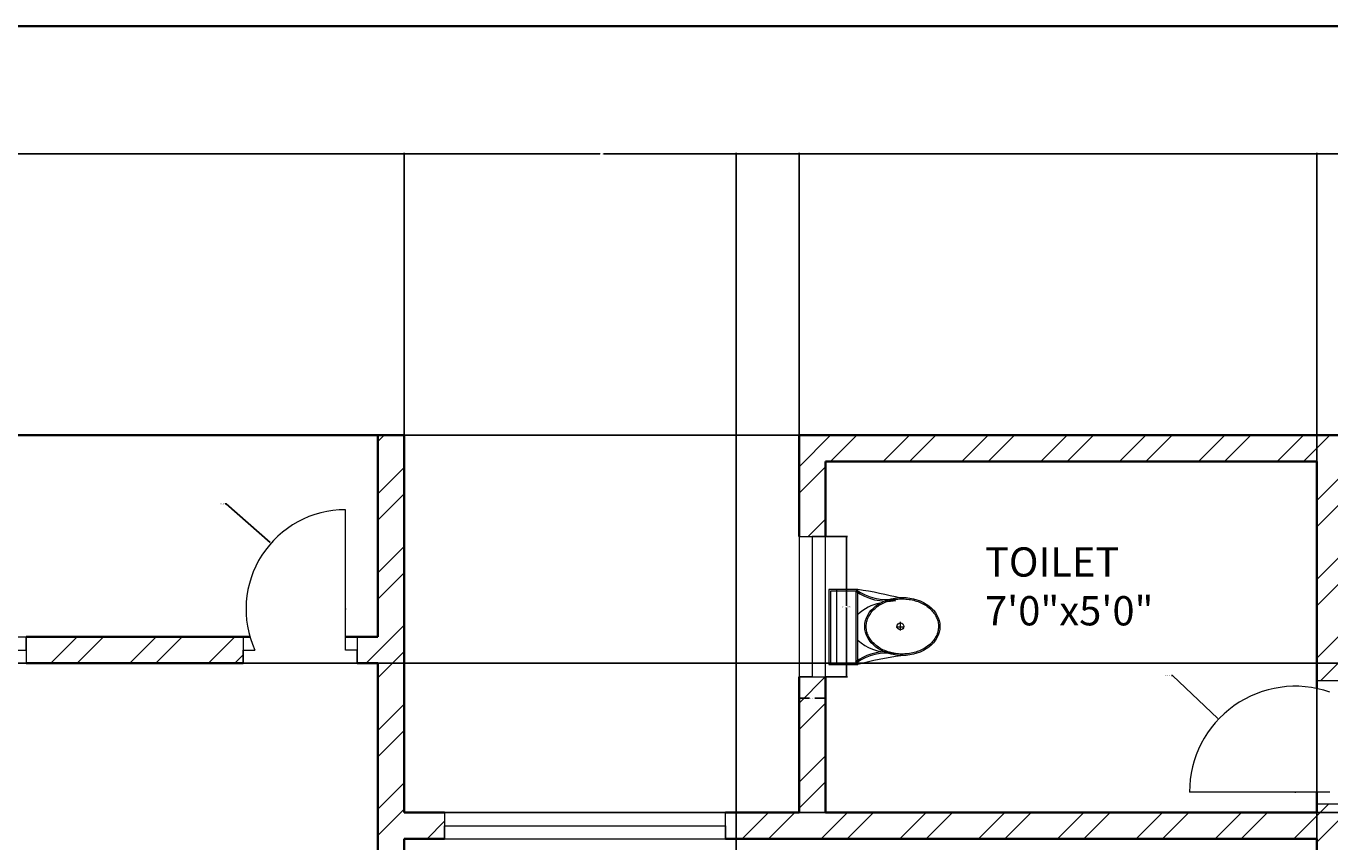
# Model space of a CAD drawing. Units: inches. Extents: x 2008 to 2657, y 1077 to 2165.
# Tile 13 of 16: x 2186 to 2409, y 2025 to 2165. Entities that reach past the tile are written whole.
import ezdxf

# ---------------------------------------------------------------- set-up
doc = ezdxf.new("R2010")
doc.units = ezdxf.units.IN
for name, color, linetype, lineweight in [('A-ANNO-DIMS', 2, 'Continuous', 18), ('A-ANNO-TTLB', 7, 'Continuous', 35), ('A-AREA-IDEN', 4, 'Continuous', 18), ('A-DOOR', 11, 'Continuous', 18), ('A-FLOR-FIXT', 8, 'Continuous', 18), ('A-GLAZ', 191, 'Continuous', 18), ('A-WALL', 7, 'Continuous', 35)]:
    doc.layers.add(name, color=color, linetype=linetype, lineweight=lineweight)
doc.layers.add('A-WALL-PATT', color=30, linetype='Continuous', lineweight=13, true_color=0xf8991e)
doc.styles.get("Standard").update_dxf_attribs({"font": 'arial.ttf'})
doc.dimstyles.get("Standard").update_dxf_attribs({"dimtxt": 0.18, "dimasz": 0.18, "dimexe": 0.18, "dimexo": 0.0625, "dimgap": 0.09, "dimtad": 0, "dimtih": 1, "dimtoh": 1, "dimdec": 4, "dimzin": 0, "dimdsep": 46, "dimtxsty": 'Standard', "dimcen": 0.09, "dimadec": 0, "dimazin": 0, "dimtfac": 1, "dimtdec": 4, "dimtofl": 0, "dimtmove": 0, "dimatfit": 3, "dimfxl": 1, "dimtolj": 1, "dimtzin": 0, "dimarcsym": 0})

# ---------------------------------------------------------------- blocks, each defined once
blk = doc.blocks.new('A$C31115884')
for p, q in [((283.1, 497.7), (223.4, 497.7)), ((257.5, 466.4), (257.5, 523.2)), ((0, 200), (0, 0)), ((520, 200), (0, 200)), ((10, 190), (10, 10)), ((510, 190), (10, 190)), ((510, 10), (510, 190)), ((520, 0), (520, 200)), ((510, 54.5), (0, 54.5)), ((10, 10), (510, 10)), ((0, 0), (520, 0))]:
    blk.add_line(p, q)
blk.add_circle((255.6, 496.4), 23.6)
for centre, radius, start, end in [((2777.7, -204.6), 2807, 165.4549, 171.71327), ((-294.5, 403.3), 364.7, 324.20913, 9.34987), ((-294.5, 403.3), 374.7, 324.20913, 9.34987), ((805.8, 403.3), 364.7, 170.65013, 215.79087), ((3237, 905), 2807, 188.28673, 194.5451), ((139.5, 406.2), 293.5, 315.84364, 2.65635), ((805.8, 403.3), 374.7, 179.20365, 215.79087), ((383.6, 406.2), 293.5, 190.27735, 224.15636)]:
    blk.add_arc(centre, radius, start, end)
blk.add_ellipse((256.2, 509.9), major_axis=(0, -260.7), ratio=0.772727)
blk.add_open_spline([(256.2, 259.2), (263.1, 259.2), (270, 259.7), (287.8, 262.3), (298.7, 265.1), (319.9, 273.1), (330.2, 278.4), (350.1, 291.1), (359.7, 298.7), (377.7, 315.9), (386.2, 325.5), (401.7, 346.6), (408.8, 358.1), (421.3, 382.5), (426.8, 395.5), (435.9, 422.4), (439.5, 436.4), (444.8, 465.1), (446.5, 479.7), (447.9, 509.2), (447.6, 524), (445, 553.3), (442.7, 567.8), (436.3, 596), (432.1, 609.7), (421.9, 636), (416, 648.6), (402.5, 672.1), (395, 683), (378.6, 703), (369.8, 712.1), (351.1, 728), (341.3, 734.8), (320.9, 746.2), (310.4, 750.7), (288.9, 757.3), (278, 759.4), (256, 761), (245, 760.6), (223.1, 757.2), (212.3, 754.3), (191.1, 746.1), (180.8, 740.7), (160.9, 727.8), (151.4, 720.1), (133.5, 702.7), (125.1, 693), (109.6, 671.7), (102.6, 660.2), (90.2, 635.7), (84.9, 622.7), (76, 595.6), (72.4, 581.6), (67.2, 552.9), (65.6, 538.2), (64.4, 508.8), (64.8, 494), (67.5, 464.7), (69.9, 450.2), (76.6, 422), (80.8, 408.3), (91.1, 382.2), (97.2, 369.7), (110.8, 346.3), (118.4, 335.4), (134.8, 315.6), (143.7, 306.7), (162.4, 290.9), (172.3, 284.2), (192.8, 273), (203.3, 268.6), (224.8, 262.2), (235.8, 260.2), (249.9, 259.3), (253, 259.2), (256.2, 259.2)], degree=3, knots=[0, 0, 0, 0, 0.110105, 0.110105, 0.285049, 0.285049, 0.459994, 0.459994, 0.634938, 0.634938, 0.809882, 0.809882, 0.984827, 0.984827, 1.159771, 1.159771, 1.334715, 1.334715, 1.50966, 1.50966, 1.684604, 1.684604, 1.859549, 1.859549, 2.034493, 2.034493, 2.209437, 2.209437, 2.384382, 2.384382, 2.559326, 2.559326, 2.73427, 2.73427, 2.909215, 2.909215, 3.084159, 3.084159, 3.259103, 3.259103, 3.434048, 3.434048, 3.608992, 3.608992, 3.783936, 3.783936, 3.958881, 3.958881, 4.133825, 4.133825, 4.30877, 4.30877, 4.483714, 4.483714, 4.658658, 4.658658, 4.833603, 4.833603, 5.008547, 5.008547, 5.183491, 5.183491, 5.358436, 5.358436, 5.53338, 5.53338, 5.708324, 5.708324, 5.883269, 5.883269, 6.058213, 6.058213, 6.233158, 6.233158, 6.283185, 6.283185, 6.283185, 6.283185])
blk = doc.blocks.new('WIN-60IN-B')
for p, q in [((0, 4.5), (0, 0)), ((0, 4.5), (60, 4.5)), ((60, 2.25), (60, 4.5)), ((60, 4.5), (60, 0)), ((0, 0), (0, 2.25)), ((0, 2.25), (60, 2.25)), ((60, 0), (0, 0))]:
    blk.add_line(p, q)
blk = doc.blocks.new('WIN-24IN-B')
for p, q in [((0, 24), (4.5, 24)), ((0, 24), (0, 0)), ((4.5, 24), (2.25, 24)), ((2.25, 24), (2.25, 0)), ((4.5, 0), (4.5, 24)), ((2.25, 0), (0, 0)), ((0, 0), (4.5, 0))]:
    blk.add_line(p, q)
blk = doc.blocks.new('*D23')
at = {"layer": 'A-ANNO-DIMS', "color": 0, "lineweight": -2, "transparency": 16777216}
for p, q in [((2322.82, 2077.34), (2326.54, 2077.34)), ((2326.36, 2077.16), (2326.36, 2065.52)), ((2326.36, 2053.52), (2326.36, 2065.16)), ((2322.82, 2053.34), (2326.54, 2053.34))]:
    blk.add_line(p, q, dxfattribs=at)
at = {"layer": 'A-ANNO-DIMS', "color": 0, "transparency": 16777216}
for points in [[(2326.33, 2077.16), (2326.39, 2077.16), (2326.36, 2077.34)], [(2326.33, 2053.52), (2326.39, 2053.52), (2326.36, 2053.34)]]:
    blk.add_solid(points, dxfattribs=at)
at = {"layer": 'Defpoints', "color": 0, "transparency": 16777216}
for p in [(2322.76, 2077.34), (2326.36, 2077.34), (2322.76, 2053.34)]:
    blk.add_point(p, dxfattribs=at)
at = {"layer": 'A-ANNO-DIMS', "color": 0, "transparency": 16777216, "insert": (2326.36, 2065.34), "char_height": 0.18, "attachment_point": 5}
blk.add_mtext('\\A1;WIN B 24 TYP.', dxfattribs=at)
blk = doc.blocks.new('*D24')
at = {"layer": 'A-ANNO-DIMS', "color": 0, "lineweight": -2, "transparency": 16777216}
for p, q in [((2318.26, 2053.28), (2318.26, 2049.56)), ((2322.76, 2053.28), (2322.76, 2049.56)), ((2318.44, 2049.74), (2320.05, 2049.74)), ((2322.58, 2049.74), (2320.97, 2049.74))]:
    blk.add_line(p, q, dxfattribs=at)
at = {"layer": 'A-ANNO-DIMS', "color": 0, "transparency": 16777216}
for points in [[(2318.44, 2049.77), (2318.44, 2049.71), (2318.26, 2049.74)], [(2322.58, 2049.77), (2322.58, 2049.71), (2322.76, 2049.74)]]:
    blk.add_solid(points, dxfattribs=at)
at = {"layer": 'Defpoints', "color": 0, "transparency": 16777216}
for p in [(2318.26, 2053.34), (2322.76, 2053.34), (2322.76, 2049.74)]:
    blk.add_point(p, dxfattribs=at)
at = {"layer": 'A-ANNO-DIMS', "color": 0, "transparency": 16777216, "insert": (2320.51, 2049.74), "char_height": 0.18, "attachment_point": 5}
blk.add_mtext('\\A1;5 TYP.', dxfattribs=at)
blk = doc.blocks.new('*D34')
at = {"layer": 'A-ANNO-DIMS', "color": 0, "lineweight": -2, "transparency": 16777216}
for p, q in [((2104.76, 2094.74), (2104.76, 2142.9)), ((2104.94, 2142.72), (2177.48, 2142.72)), ((2250.58, 2142.72), (2178.04, 2142.72)), ((2250.76, 2094.74), (2250.76, 2142.9))]:
    blk.add_line(p, q, dxfattribs=at)
at = {"layer": 'A-ANNO-DIMS', "color": 0, "transparency": 16777216}
for points in [[(2104.94, 2142.75), (2104.94, 2142.69), (2104.76, 2142.72)], [(2250.58, 2142.75), (2250.58, 2142.69), (2250.76, 2142.72)]]:
    blk.add_solid(points, dxfattribs=at)
at = {"layer": 'Defpoints', "color": 0, "transparency": 16777216}
for p in [(2250.76, 2142.72), (2104.76, 2094.67), (2250.76, 2094.67)]:
    blk.add_point(p, dxfattribs=at)
at = {"layer": 'A-ANNO-DIMS', "color": 0, "transparency": 16777216, "insert": (2177.76, 2142.72), "char_height": 0.18, "attachment_point": 5}
blk.add_mtext('\\A1;146', dxfattribs=at)
blk = doc.blocks.new('*D35')
at = {"layer": 'A-ANNO-DIMS', "color": 0, "lineweight": -2, "transparency": 16777216}
for p, q in [((2250.76, 2094.74), (2250.76, 2142.9)), ((2250.94, 2142.72), (2284.19, 2142.72)), ((2318.08, 2142.72), (2284.84, 2142.72)), ((2318.26, 2094.74), (2318.26, 2142.9))]:
    blk.add_line(p, q, dxfattribs=at)
at = {"layer": 'A-ANNO-DIMS', "color": 0, "transparency": 16777216}
for points in [[(2250.94, 2142.75), (2250.94, 2142.69), (2250.76, 2142.72)], [(2318.08, 2142.75), (2318.08, 2142.69), (2318.26, 2142.72)]]:
    blk.add_solid(points, dxfattribs=at)
at = {"layer": 'Defpoints', "color": 0, "transparency": 16777216}
for p in [(2318.26, 2142.72), (2250.76, 2094.67), (2318.26, 2094.67)]:
    blk.add_point(p, dxfattribs=at)
at = {"layer": 'A-ANNO-DIMS', "color": 0, "transparency": 16777216, "insert": (2284.51, 2142.72), "char_height": 0.18, "attachment_point": 5}
blk.add_mtext('\\A1;67.5', dxfattribs=at)
blk = doc.blocks.new('*D36')
at = {"layer": 'A-ANNO-DIMS', "color": 0, "lineweight": -2, "transparency": 16777216}
for p, q in [((2318.26, 2094.74), (2318.26, 2142.9)), ((2318.44, 2142.72), (2364.54, 2142.72)), ((2411.08, 2142.72), (2364.98, 2142.72)), ((2411.26, 2094.74), (2411.26, 2142.9))]:
    blk.add_line(p, q, dxfattribs=at)
at = {"layer": 'A-ANNO-DIMS', "color": 0, "transparency": 16777216}
for points in [[(2318.44, 2142.75), (2318.44, 2142.69), (2318.26, 2142.72)], [(2411.08, 2142.75), (2411.08, 2142.69), (2411.26, 2142.72)]]:
    blk.add_solid(points, dxfattribs=at)
at = {"layer": 'Defpoints', "color": 0, "transparency": 16777216}
for p in [(2411.26, 2142.72), (2318.26, 2094.67), (2411.26, 2094.67)]:
    blk.add_point(p, dxfattribs=at)
at = {"layer": 'A-ANNO-DIMS', "color": 0, "transparency": 16777216, "insert": (2364.76, 2142.72), "char_height": 0.18, "attachment_point": 5}
blk.add_mtext('\\A1;93', dxfattribs=at)
blk = doc.blocks.new('*D49')
at = {"layer": 'A-ANNO-DIMS', "color": 0, "lineweight": -2, "transparency": 16777216}
for p, q in [((2250.82, 2094.67), (2624.99, 2094.67)), ((2624.81, 2094.49), (2624.81, 2062.61)), ((2624.81, 2030.35), (2624.81, 2062.24)), ((2250.82, 2030.17), (2624.99, 2030.17))]:
    blk.add_line(p, q, dxfattribs=at)
at = {"layer": 'A-ANNO-DIMS', "color": 0, "transparency": 16777216}
for points in [[(2624.78, 2094.49), (2624.84, 2094.49), (2624.81, 2094.67)], [(2624.78, 2030.35), (2624.84, 2030.35), (2624.81, 2030.17)]]:
    blk.add_solid(points, dxfattribs=at)
at = {"layer": 'Defpoints', "color": 0, "transparency": 16777216}
for p in [(2250.76, 2094.67), (2624.81, 2094.67), (2250.76, 2030.17)]:
    blk.add_point(p, dxfattribs=at)
at = {"layer": 'A-ANNO-DIMS', "color": 0, "transparency": 16777216, "insert": (2624.81, 2062.42), "char_height": 0.18, "attachment_point": 5}
blk.add_mtext('\\A1;64.5', dxfattribs=at)
blk = doc.blocks.new('*D51')
at = {"layer": 'A-ANNO-DIMS', "color": 0, "lineweight": -2, "transparency": 16777216}
for p, q in [((2307.5, 1617.74), (2307.5, 2142.9)), ((2307.68, 2142.72), (2356.74, 2142.72)), ((2406.58, 2142.72), (2357.53, 2142.72)), ((2406.76, 1617.74), (2406.76, 2142.9))]:
    blk.add_line(p, q, dxfattribs=at)
at = {"layer": 'A-ANNO-DIMS', "color": 0, "transparency": 16777216}
for points in [[(2307.68, 2142.75), (2307.68, 2142.69), (2307.5, 2142.72)], [(2406.58, 2142.75), (2406.58, 2142.69), (2406.76, 2142.72)]]:
    blk.add_solid(points, dxfattribs=at)
at = {"layer": 'Defpoints', "color": 0, "transparency": 16777216}
for p in [(2406.76, 2142.72), (2307.5, 1617.67), (2406.76, 1617.67)]:
    blk.add_point(p, dxfattribs=at)
at = {"layer": 'A-ANNO-DIMS', "color": 0, "transparency": 16777216, "insert": (2357.13, 2142.72), "char_height": 0.18, "attachment_point": 5}
blk.add_mtext('\\A1;99.26', dxfattribs=at)
blk = doc.blocks.new('*D66')
at = {"layer": 'A-ANNO-DIMS', "color": 0, "lineweight": -2, "transparency": 16777216}
for p, q in [((2572.2, 2055.67), (2028.03, 2055.67)), ((2028.21, 2055.49), (2028.21, 2025.16)), ((2028.21, 1994.47), (2028.21, 2024.8)), ((2572.2, 1994.29), (2028.03, 1994.29))]:
    blk.add_line(p, q, dxfattribs=at)
at = {"layer": 'A-ANNO-DIMS', "color": 0, "transparency": 16777216}
for points in [[(2028.18, 2055.49), (2028.24, 2055.49), (2028.21, 2055.67)], [(2028.18, 1994.47), (2028.24, 1994.47), (2028.21, 1994.29)]]:
    blk.add_solid(points, dxfattribs=at)
at = {"layer": 'Defpoints', "color": 0, "transparency": 16777216}
for p in [(2572.26, 2055.67), (2028.21, 1994.29), (2572.26, 1994.29)]:
    blk.add_point(p, dxfattribs=at)
at = {"layer": 'A-ANNO-DIMS', "color": 0, "transparency": 16777216, "insert": (2028.21, 2024.98), "char_height": 0.18, "attachment_point": 5}
blk.add_mtext('\\A1;61.39', dxfattribs=at)
blk = doc.blocks.new('*D85')
at = {"layer": 'A-ANNO-DIMS', "color": 0, "lineweight": -2, "transparency": 16777216}
for p, q in [((2220.17, 2082.93), (2220.35, 2082.93)), ((2220.35, 2082.93), (2227.86, 2076.3)), ((2240.63, 2064.94), (2240.81, 2064.94)), ((2240.72, 2064.85), (2240.72, 2065.03))]:
    blk.add_line(p, q, dxfattribs=at)
at = {"layer": 'A-ANNO-DIMS', "color": 0, "transparency": 16777216}
blk.add_solid([(2227.88, 2076.33), (2227.84, 2076.28), (2227.99, 2076.18)], dxfattribs=at)
at = {"layer": 'Defpoints', "color": 0, "transparency": 16777216}
for p in [(2227.99, 2076.18), (2240.72, 2064.94)]:
    blk.add_point(p, dxfattribs=at)
at = {"layer": 'A-ANNO-DIMS', "color": 0, "transparency": 16777216, "insert": (2219.69, 2082.93), "char_height": 0.18, "attachment_point": 5}
blk.add_mtext('\\A1;R16.99', dxfattribs=at)
blk = doc.blocks.new('*D86')
at = {"layer": 'A-ANNO-DIMS', "color": 0, "lineweight": -2, "transparency": 16777216}
for p, q in [((2381.93, 2053.59), (2382.11, 2053.59)), ((2382.11, 2053.59), (2389.85, 2046.24)), ((2403, 2033.67), (2403.18, 2033.67)), ((2403.09, 2033.58), (2403.09, 2033.76))]:
    blk.add_line(p, q, dxfattribs=at)
at = {"layer": 'A-ANNO-DIMS', "color": 0, "transparency": 16777216}
blk.add_solid([(2389.87, 2046.27), (2389.83, 2046.22), (2389.98, 2046.12)], dxfattribs=at)
at = {"layer": 'Defpoints', "color": 0, "transparency": 16777216}
for p in [(2389.98, 2046.12), (2403.09, 2033.67)]:
    blk.add_point(p, dxfattribs=at)
at = {"layer": 'A-ANNO-DIMS', "color": 0, "transparency": 16777216, "insert": (2381.38, 2053.59), "char_height": 0.18, "attachment_point": 5}
blk.add_mtext('\\A1;R18.076', dxfattribs=at)

msp = doc.modelspace()

# ---------------------------------------------------------------- hatches: boundary and pattern name
at = {"layer": 'A-WALL-PATT'}
h = msp.add_hatch(dxfattribs=at)
h.set_pattern_fill('ANSI32', color=256)
h.paths.add_polyline_path([(2109.2619, 2094.6743), (2104.7619, 2094.6743), (2104.7619, 2072.1743), (2104.7619, 2021.6151), (2109.2619, 2021.6151), (2109.2619, 2055.6743), (2126.1387, 2055.6743), (2126.1387, 2057.9243), (2126.1387, 2060.1743), (2109.2619, 2060.1743)])
h.paths.add_polyline_path([(2223.2494, 2057.9243), (2223.2494, 2060.1743), (2186.1387, 2060.1743), (2186.1387, 2055.6743), (2223.2494, 2055.6743)])
h.paths.add_polyline_path([(2250.7619, 2072.1743), (2250.7619, 2090.1743), (2250.7619, 2094.6743), (2246.2619, 2094.6743), (2246.2619, 2060.1743), (2242.7242, 2060.1743), (2242.7242, 2055.6743), (2246.2619, 2055.6743), (2246.2619, 1899.6743), (2242.7458, 1899.6743), (2242.7458, 1897.4243), (2242.7458, 1895.1743), (2246.2619, 1895.1743), (2246.2619, 1878.8745), (2248.5119, 1878.8745), (2250.7619, 1878.8745), (2250.7619, 1991.1743), (2250.7619, 2025.6743), (2257.6798, 2025.6743), (2257.6798, 2027.9243), (2257.6798, 2030.1743), (2250.7619, 2030.1743)])
h.paths.add_polyline_path([(2411.2619, 2031.6743), (2409.0119, 2031.6743), (2406.7619, 2031.6743), (2406.7619, 2030.1743), (2322.7619, 2030.1743), (2322.7619, 2053.3443), (2318.2619, 2053.3443), (2318.2619, 2030.1743), (2305.6798, 2030.1743), (2305.6798, 2025.6743), (2318.2619, 2025.6743), (2322.7619, 2025.6743), (2406.7619, 2025.6743), (2406.7619, 1995.6743), (2406.7619, 1847.2677), (2250.7619, 1847.2677), (2250.7619, 1850.9902), (2248.5119, 1850.9902), (2246.2619, 1850.9902), (2246.2619, 1847.1743), (2246.2619, 1842.7677), (2303.0015, 1842.7677), (2303.0015, 1667.2413), (2298.4208, 1667.2413), (2298.4208, 1662.7413), (2303.0015, 1662.7413), (2303.0015, 1649.8758), (2307.5015, 1649.8758), (2307.5015, 1842.7677), (2406.7619, 1842.7677), (2411.2619, 1842.7677), (2411.2619, 1878.6743), (2415.8196, 1878.6743), (2415.8196, 1880.9243), (2415.8196, 1883.1743), (2411.2619, 1883.1743)])
h.paths.add_polyline_path([(2411.2619, 2094.6743), (2406.7619, 2094.6743), (2318.2619, 2094.6743), (2318.2619, 2077.3443), (2322.7619, 2077.3443), (2322.7619, 2090.1743), (2406.7619, 2090.1743), (2406.7619, 2072.1743), (2406.7619, 2067.6743), (2406.7619, 2052.7524), (2411.2619, 2052.7524), (2411.2619, 2055.6743), (2414.9888, 2055.6743), (2414.9888, 2057.9243), (2414.9888, 2060.1743), (2411.2619, 2060.1743), (2411.2619, 2072.1743)])
h.paths.add_polyline_path([(2576.7619, 2072.1743), (2576.7619, 2094.6743), (2572.2619, 2094.6743), (2572.2619, 2060.1743), (2525.8113, 2060.1743), (2525.8113, 2055.6743), (2572.2619, 2055.6743), (2572.2619, 1994.289), (2576.7619, 1994.289)])
h.paths.add_polyline_path([(2465.8113, 2060.1743), (2436.2802, 2060.1743), (2436.2802, 2055.6743), (2465.8113, 2055.6743), (2465.8113, 2057.9243)])
h.paths.add_polyline_path([(2576.7619, 1934.289), (2574.5119, 1934.289), (2572.2619, 1934.289), (2572.2619, 1883.1743), (2447.7027, 1883.1743), (2447.7027, 1878.6743), (2459.7619, 1878.6743), (2459.7619, 1830.4982), (2464.2619, 1830.4982), (2464.2619, 1878.6743), (2572.2619, 1878.6743), (2572.2619, 1868.4883), (2576.7619, 1868.4883)])
h.paths.add_polyline_path([(2576.7619, 1832.4883), (2572.2619, 1832.4883), (2572.2619, 1806.6743), (2464.2619, 1806.6743), (2464.2619, 1809.6629), (2459.7619, 1809.6629), (2459.7619, 1802.1743), (2483.7619, 1802.1743), (2483.7619, 1778.1743), (2488.2619, 1778.1743), (2488.2619, 1802.1743), (2572.2619, 1802.1743), (2572.2619, 1793.6101), (2576.7619, 1793.6101)])
h.paths.add_polyline_path([(2576.7619, 1769.6101), (2572.2619, 1769.6101), (2572.2619, 1754.1743), (2488.2619, 1754.1743), (2488.2619, 1757.2675), (2486.0119, 1757.2675), (2483.7619, 1757.2675), (2483.7619, 1754.1743), (2447.4528, 1754.1743), (2447.4528, 1749.6743), (2483.7619, 1749.6743), (2572.2619, 1749.6743), (2572.2619, 1715.1837), (2576.7619, 1715.1837)])
h.paths.add_polyline_path([(2576.7619, 1655.1837), (2572.2619, 1655.1837), (2572.2619, 1617.6743), (2411.2619, 1617.6743), (2411.2619, 1749.6743), (2414.2827, 1749.6743), (2414.2827, 1754.1743), (2406.7619, 1754.1743), (2406.7619, 1749.6743), (2406.7619, 1617.6743), (2307.5015, 1617.6743), (2307.5015, 1621.0007), (2305.2515, 1621.0007), (2303.0015, 1621.0007), (2303.0015, 1609.6944), (2307.5015, 1609.6944), (2307.5015, 1613.1743), (2406.7619, 1613.1743), (2406.7619, 1476.6743), (2415.532, 1476.6743), (2415.532, 1478.9243), (2415.532, 1481.1743), (2411.2619, 1481.1743), (2411.2619, 1613.1743), (2572.2619, 1613.1743), (2572.2619, 1584.6086), (2576.7619, 1584.6086)])
h.paths.add_polyline_path([(2576.7619, 1524.6086), (2572.2619, 1524.6086), (2572.2619, 1481.1743), (2483.7619, 1481.1743), (2447.5119, 1481.1743), (2447.5119, 1476.6743), (2483.7619, 1476.6743), (2483.7619, 1473.5051), (2488.2619, 1473.5051), (2488.2619, 1476.6743), (2572.2619, 1476.6743), (2572.2619, 1469.5488), (2576.7619, 1469.5488)])
h.paths.add_polyline_path([(2576.7619, 1445.5488), (2572.2619, 1445.5488), (2572.2619, 1428.6743), (2488.2619, 1428.6743), (2488.2619, 1455.6743), (2486.0119, 1455.6743), (2483.7619, 1455.6743), (2483.7619, 1428.6743), (2459.7619, 1428.6743), (2459.7619, 1422.1519), (2464.2619, 1422.1519), (2464.2619, 1424.1743), (2572.2619, 1424.1743), (2572.2619, 1407.5685), (2576.7619, 1407.5685)])
h.paths.add_polyline_path([(2576.7619, 1371.5685), (2572.2619, 1371.5685), (2572.2619, 1352.1743), (2464.2619, 1352.1743), (2464.2619, 1403.1384), (2462.0119, 1403.1384), (2459.7619, 1403.1384), (2459.7619, 1352.1743), (2446.3194, 1352.1743), (2446.3194, 1347.6743), (2572.2619, 1347.6743), (2572.2619, 1321.0291), (2576.7619, 1321.0291)])
h.paths.add_polyline_path([(2462.703, 1227.6743), (2436.0298, 1227.6743), (2436.0298, 1225.4243), (2436.0298, 1223.1743), (2462.703, 1223.1743), (2462.703, 1225.4243)])
h.paths.add_polyline_path([(2576.7619, 1261.0291), (2574.5119, 1261.0291), (2572.2619, 1261.0291), (2572.2619, 1227.6743), (2522.703, 1227.6743), (2522.703, 1223.1743), (2572.2619, 1223.1743), (2572.2619, 1188.6743), (2576.7619, 1188.6743), (2576.7619, 1193.1743), (2576.7619, 1223.1743)])
h.paths.add_polyline_path([(2414.2823, 1227.6743), (2411.2619, 1227.6743), (2411.2619, 1267.1779), (2409.0119, 1267.1779), (2406.7619, 1267.1779), (2406.7619, 1227.6743), (2322.7619, 1227.6743), (2322.7619, 1244.3623), (2318.2619, 1244.3623), (2318.2619, 1223.1743), (2406.7619, 1223.1743), (2406.7619, 1193.1743), (2406.7619, 1188.6743), (2411.2619, 1188.6743), (2411.2619, 1193.1743), (2411.2619, 1223.1743), (2414.2823, 1223.1743)])
h.paths.add_polyline_path([(2411.2619, 1347.6743), (2414.702, 1347.6743), (2414.702, 1349.9243), (2414.702, 1352.1743), (2411.2619, 1352.1743), (2411.2619, 1416.7413), (2307.5015, 1416.7413), (2307.5015, 1579.8489), (2305.2515, 1579.8489), (2303.0015, 1579.8489), (2303.0015, 1566.7413), (2299.2719, 1566.7413), (2299.2719, 1562.2413), (2303.0015, 1562.2413), (2303.0015, 1416.7413), (2246.2619, 1416.7413), (2246.2619, 1409.8616), (2250.7619, 1409.8616), (2250.7619, 1412.2413), (2406.7619, 1412.2413), (2406.7619, 1292.1743), (2304.9703, 1292.1743), (2304.9703, 1287.6743), (2318.2619, 1287.6743), (2318.2619, 1268.3623), (2322.7619, 1268.3623), (2322.7619, 1287.6743), (2406.7619, 1287.6743), (2406.7619, 1285.4748), (2411.2619, 1285.4748)])
h.paths.add_polyline_path([(2109.2619, 1262.7482), (2104.7619, 1262.7482), (2104.7619, 1223.1743), (2104.7619, 1193.1743), (2104.7619, 1188.6743), (2109.2619, 1188.6743), (2109.2619, 1223.1743), (2126.7928, 1223.1743), (2126.7928, 1225.4243), (2126.7928, 1227.6743), (2109.2619, 1227.6743)])
h.paths.add_polyline_path([(2222.3268, 1227.6743), (2186.7928, 1227.6743), (2186.7928, 1223.1743), (2222.3268, 1223.1743)])
h.paths.add_polyline_path([(2250.7619, 1287.6743), (2256.9703, 1287.6743), (2256.9703, 1289.9243), (2256.9703, 1292.1743), (2250.7619, 1292.1743), (2250.7619, 1382.2078), (2248.5119, 1382.2078), (2246.2619, 1382.2078), (2246.2619, 1347.6743), (2246.2619, 1227.6743), (2242.6068, 1227.6743), (2242.6068, 1223.1743), (2246.2619, 1223.1743), (2246.2619, 1188.6743), (2250.7619, 1188.6743), (2250.7619, 1193.1743), (2250.7619, 1227.6743)])
h.paths.add_polyline_path([(2133.2619, 1349.9243), (2133.2619, 1352.1743), (2109.2619, 1352.1743), (2109.2619, 1375.2826), (2104.7619, 1375.2826), (2104.7619, 1322.7482), (2109.2619, 1322.7482), (2109.2619, 1347.6743), (2133.2619, 1347.6743)])
h.paths.add_polyline_path([(2210.2105, 1352.1743), (2161.7619, 1352.1743), (2161.7619, 1412.2413), (2185.7619, 1412.2413), (2185.7619, 1420.1851), (2183.5119, 1420.1851), (2181.2619, 1420.1851), (2181.2619, 1416.7413), (2109.2619, 1416.7413), (2109.2619, 1452.4006), (2104.7619, 1452.4006), (2104.7619, 1399.2826), (2109.2619, 1399.2826), (2109.2619, 1412.2413), (2157.2619, 1412.2413), (2157.2619, 1352.1743), (2154.3383, 1352.1743), (2154.3383, 1347.6743), (2210.2105, 1347.6743)])
h.paths.add_polyline_path([(2185.7619, 1514.2413), (2161.7619, 1514.2413), (2161.7619, 1518.1307), (2159.5119, 1518.1307), (2157.2619, 1518.1307), (2157.2619, 1514.2413), (2109.2619, 1514.2413), (2109.2619, 1528.997), (2107.0119, 1528.997), (2104.7619, 1528.997), (2104.7619, 1488.4006), (2109.2619, 1488.4006), (2109.2619, 1509.7413), (2181.2619, 1509.7413), (2181.2619, 1441.2042), (2185.7619, 1441.2042)])
h.paths.add_polyline_path([(2270.4025, 1566.7413), (2109.2619, 1566.7413), (2080.7619, 1566.7413), (2080.7619, 1586.5643), (2076.2619, 1586.5643), (2076.2619, 1562.2413), (2080.7619, 1562.2413), (2104.7619, 1562.2413), (2104.7619, 1552.997), (2109.2619, 1552.997), (2109.2619, 1562.2413), (2157.2619, 1562.2413), (2157.2619, 1538.2413), (2161.7619, 1538.2413), (2161.7619, 1562.2413), (2205.2619, 1562.2413), (2270.4025, 1562.2413)])
h.paths.add_polyline_path([(2131.6813, 1897.4243), (2131.6813, 1899.6743), (2109.2619, 1899.6743), (2109.2619, 1961.6151), (2104.7619, 1961.6151), (2104.7619, 1886.8042), (2109.2619, 1886.8042), (2109.2619, 1895.1743), (2131.6813, 1895.1743)])
h.paths.add_polyline_path([(2185.7619, 1847.1743), (2161.7619, 1847.1743), (2161.7619, 1895.1743), (2185.7619, 1895.1743), (2211.543, 1895.1743), (2211.543, 1897.4243), (2211.543, 1899.6743), (2154.0916, 1899.6743), (2154.0916, 1897.4243), (2154.0916, 1895.1743), (2157.2619, 1895.1743), (2157.2619, 1847.1743), (2109.2619, 1847.1743), (2109.2619, 1862.8042), (2104.7619, 1862.8042), (2104.7619, 1821.243), (2109.2619, 1821.243), (2109.2619, 1842.6743), (2181.2619, 1842.6743), (2181.2619, 1840.6763), (2185.7619, 1840.6763)])
h.paths.add_polyline_path([(2109.2619, 1785.243), (2104.7619, 1785.243), (2104.7619, 1715.4691), (2109.2619, 1715.4691), (2109.2619, 1730.8423), (2157.2619, 1730.8423), (2157.2619, 1727.6404), (2161.7619, 1727.6404), (2161.7619, 1730.8423), (2185.7619, 1730.8423), (2185.7619, 1822.1438), (2183.5119, 1822.1438), (2181.2619, 1822.1438), (2181.2619, 1735.3423), (2109.2619, 1735.3423)])
h.paths.add_polyline_path([(2109.2619, 1691.4691), (2104.7619, 1691.4691), (2104.7619, 1667.2413), (2076.2619, 1667.2413), (2076.2619, 1646.5643), (2080.7619, 1646.5643), (2080.7619, 1662.7413), (2109.2619, 1662.7413), (2271.4941, 1662.7413), (2271.4941, 1664.9913), (2271.4941, 1667.2413), (2181.2619, 1667.2413), (2161.7619, 1667.2413), (2161.7619, 1708.3752), (2159.5119, 1708.3752), (2157.2619, 1708.3752), (2157.2619, 1667.2413), (2109.2619, 1667.2413)])
h.paths.add_polyline_path([(2233.1467, 1747.4973), (2270.0737, 1747.4973), (2270.0737, 1766.1547), (2233.1467, 1766.1547)], flags=9)

# ---------------------------------------------------------------- linework, layer by layer
at = {"layer": 'A-ANNO-TTLB'}
msp.add_lwpolyline([(2008.4537, 2164.5615), (2657.4477, 2164.5615), (2657.4477, 1076.8888), (2008.4537, 1076.8888)], close=True, dxfattribs=at)
at = {"layer": 'A-DOOR'}
for p, q in [((2240.7242, 2057.9243), (2240.7242, 2081.9243)), ((2223.2494, 2060.1743), (2223.2494, 2055.6743)), ((2242.7242, 2060.1743), (2242.7242, 2055.6743)), ((2223.2494, 2055.6743), (2223.2494, 2057.9243)), ((2223.2494, 2057.9243), (2225.2494, 2057.9243)), ((2242.7242, 2057.9243), (2240.7242, 2057.9243)), ((2242.7242, 2055.6743), (2242.7242, 2057.9243)), ((2406.7619, 2052.7524), (2411.2619, 2052.7524)), ((2409.0119, 2033.6743), (2385.0119, 2033.6743)), ((2406.7619, 2031.6743), (2411.2619, 2031.6743))]:
    msp.add_line(p, q, dxfattribs=at)
for centre, radius, start, end in [((2240.7242, 2064.9354), 16.989, 90, 204.373471), ((2403.0881, 2033.6743), 18.0762, 70.87007, 180)]:
    msp.add_arc(centre, radius, start, end, dxfattribs=at)
at = {"layer": 'A-GLAZ'}
for p, q in [((2257.6798, 2030.1743), (2257.6798, 2025.6743)), ((2305.6798, 2030.1743), (2257.6798, 2030.1743)), ((2305.6798, 2025.6743), (2305.6798, 2030.1743)), ((2257.6798, 2025.6743), (2257.6798, 2027.9243)), ((2257.6798, 2027.9243), (2305.6798, 2027.9243)), ((2305.6798, 2027.9243), (2305.6798, 2025.6743)), ((2257.6798, 2025.6743), (2305.6798, 2025.6743))]:
    msp.add_line(p, q, dxfattribs=at)
at = {"layer": 'A-WALL'}
for p, q in [((2250.7619, 2094.6743), (2104.7619, 2094.6743)), ((2246.2619, 2094.6743), (2246.2619, 2060.1743)), ((2250.7619, 2094.6743), (2246.2619, 2094.6743)), ((2250.7619, 2090.1743), (2250.7619, 2094.6743)), ((2406.7619, 2094.6743), (2318.2619, 2094.6743)), ((2318.2619, 2077.3443), (2318.2619, 2094.6743)), ((2406.7619, 2094.6743), (2572.2619, 2094.6743)), ((2250.7619, 2072.1743), (2250.7619, 2090.1743)), ((2322.7619, 2090.1743), (2322.7619, 2077.3443)), ((2322.7619, 2090.1743), (2406.7619, 2090.1743)), ((2406.7619, 2072.1743), (2406.7619, 2090.1743)), ((2246.2619, 2072.1743), (2246.2619, 2060.1743)), ((2250.7619, 2072.1743), (2250.7619, 2030.1743)), ((2406.7619, 2067.6743), (2406.7619, 2072.1743)), ((2406.7619, 2067.6743), (2406.7619, 2051.3733)), ((2186.1387, 2060.1743), (2224.416, 2060.1743)), ((2240.7242, 2060.1743), (2246.2619, 2060.1743)), ((2186.1387, 2055.6743), (2223.2494, 2055.6743)), ((2242.7242, 2055.6743), (2246.2619, 2055.6743)), ((2246.2619, 2055.6743), (2246.2619, 1899.6743)), ((2318.2619, 2030.1743), (2318.2619, 2053.3443)), ((2322.7619, 2053.3443), (2322.7619, 2030.1743)), ((2406.7619, 2033.6743), (2406.7619, 2030.1743)), ((2257.6798, 2030.1743), (2250.7619, 2030.1743)), ((2318.2619, 2030.1743), (2305.6798, 2030.1743)), ((2322.7619, 2030.1743), (2406.7619, 2030.1743)), ((2250.7619, 2025.6743), (2250.7619, 1877.7035)), ((2257.6798, 2025.6743), (2250.7619, 2025.6743)), ((2318.2619, 2025.6743), (2305.6798, 2025.6743)), ((2322.7619, 2025.6743), (2318.2619, 2025.6743)), ((2406.7619, 2025.6743), (2322.7619, 2025.6743)), ((2406.7619, 2025.6743), (2406.7619, 1995.6743))]:
    msp.add_line(p, q, dxfattribs=at)

# ---------------------------------------------------------------- block references
at = {"layer": 'A-FLOR-FIXT', "xscale": 0.0246256636748975, "yscale": 0.0246256636748975, "zscale": 0.0246256636748975, "rotation": 270}
msp.add_blockref('A$C31115884', (2323.3687, 2068.2761), dxfattribs=at)
at = {"layer": 'A-GLAZ'}
for name, p in [('WIN-24IN-B', (2318.262, 2053.344)), ('WIN-60IN-B', (2126.139, 2055.674))]:
    msp.add_blockref(name, p, dxfattribs=at)

# ---------------------------------------------------------------- texts
at = {"layer": 'A-AREA-IDEN', "insert": (2350.0509, 2075.4874), "char_height": 5, "attachment_point": 1}
msp.add_mtext_dynamic_manual_height_columns('TOILET\\P7\'0"x5\'0"', width=100.78829, gutter_width=12.5, heights=[0], dxfattribs=at)

# ---------------------------------------------------------------- dimensions: what is measured, and where the dimension line sits
at = {"layer": 'A-ANNO-DIMS'}
for base, p1, p2, override, picture, middle in [((2250.7619, 2142.7243), (2104.7619, 2094.6743), (2250.7619, 2094.6743), {"dimdec": 0, "dimlfac": 1, "dimrnd": 0, "dimzin": 0, "dimdsep": 46, "dimlunit": 2}, '*D34', (2177.7619, 2142.7243)), ((2318.2619, 2142.7243), (2250.7619, 2094.6743), (2318.2619, 2094.6743), {"dimdec": 1, "dimlfac": 1, "dimrnd": 0, "dimzin": 0, "dimdsep": 46, "dimlunit": 2}, '*D35', (2284.5119, 2142.7243)), ((2406.7619, 2142.7243), (2307.5015, 1617.6743), (2406.7619, 1617.6743), {"dimdec": 2, "dimlfac": 1, "dimrnd": 0, "dimzin": 0, "dimdsep": 46, "dimlunit": 2}, '*D51', (2357.1317, 2142.7243)), ((2411.2619, 2142.7243), (2318.2619, 2094.6743), (2411.2619, 2094.6743), {"dimdec": 0, "dimlfac": 1, "dimrnd": 0, "dimzin": 0, "dimdsep": 46, "dimlunit": 2}, '*D36', (2364.7619, 2142.7243))]:
    dim = msp.add_linear_dim(base=base, p1=p1, p2=p2, dimstyle='Standard', override=override, dxfattribs=at)
    dim.commit()
    dim.dimension.update_dxf_attribs({"geometry": picture, "text_midpoint": middle})
for base, p1, p2, override, picture, middle in [((2624.8119, 2094.6743), (2250.7619, 2030.1743), (2250.7619, 2094.6743), {"dimdec": 1, "dimlfac": 1, "dimrnd": 0, "dimzin": 0, "dimdsep": 46, "dimlunit": 2}, '*D49', (2624.8119, 2062.4243)), ((2028.2119, 1994.289), (2572.2619, 2055.6743), (2572.2619, 1994.289), {"dimdec": 2, "dimlfac": 1, "dimrnd": 0, "dimzin": 0, "dimdsep": 46, "dimlunit": 2}, '*D66', (2028.2119, 2024.9817))]:
    dim = msp.add_linear_dim(base=base, p1=p1, p2=p2, angle=90, dimstyle='Standard', override=override, dxfattribs=at)
    dim.commit()
    dim.dimension.update_dxf_attribs({"geometry": picture, "text_midpoint": middle})
for center, mpoint, override, picture, middle in [((2240.7242, 2064.9354), (2227.9922, 2076.1835), {"dimdec": 2, "dimlfac": 1, "dimrnd": 0, "dimzin": 0, "dimdsep": 46, "dimlunit": 2}, '*D85', (2219.693, 2082.9324)), ((2403.0881, 2033.6743), (2389.9788, 2046.1201), {"dimdec": 3, "dimlfac": 1, "dimrnd": 0, "dimzin": 0, "dimdsep": 46, "dimlunit": 2}, '*D86', (2381.3836, 2053.5875))]:
    dim = msp.add_radius_dim(center=center, mpoint=mpoint, dimstyle='Standard', override=override, dxfattribs=at)
    dim.commit()
    dim.dimension.update_dxf_attribs({"geometry": picture, "text_midpoint": middle, "dimtype": 164})
dim = msp.add_linear_dim(base=(2326.3619, 2077.3443), p1=(2322.7619, 2053.3443), p2=(2322.7619, 2077.3443), angle=90, text='WIN B <> TYP.', dimstyle='Standard', override={"dimdec": 0, "dimlfac": 1, "dimrnd": 0, "dimzin": 0, "dimdsep": 46, "dimlunit": 2}, dxfattribs=at)
dim.commit()
dim.dimension.update_dxf_attribs({"geometry": '*D23', "text_midpoint": (2326.3619, 2065.3443)})
dim = msp.add_linear_dim(base=(2322.7619004523, 2049.7442964476), p1=(2318.2619004523, 2053.3442964476), p2=(2322.7619004523, 2053.3442964476), text='<> TYP.', dimstyle='Standard', override={"dimdec": 0, "dimlfac": 1, "dimrnd": 0, "dimzin": 0, "dimdsep": 46, "dimlunit": 2}, dxfattribs=at)
dim.commit()
dim.dimension.update_dxf_attribs({"geometry": '*D24', "text_midpoint": (2320.5119004523, 2049.7442964476)})

doc.saveas('drawing.dxf')
